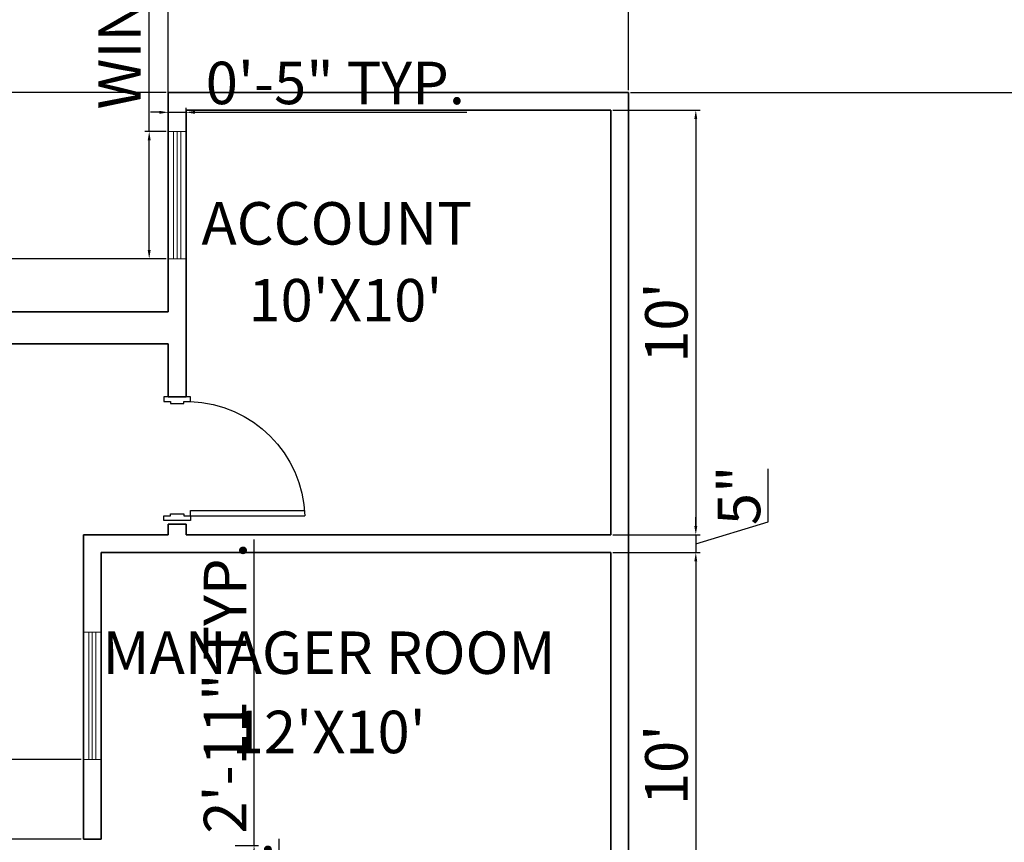
# Model space of a CAD drawing. Units: inches. Extents: x 2319 to 3765, y 2872 to 3950.
# Tile 7 of 9: x 2783 to 3061, y 3357 to 3589. Entities that reach past the tile are written whole.
import ezdxf

# ---------------------------------------------------------------- set-up
doc = ezdxf.new("R2010")
doc.units = ezdxf.units.IN
for name, color, linetype, lineweight in [('A-ANNO-DIMS', 2, 'Continuous', 18), ('A-AREA-IDEN', 7, 'Continuous', 18), ('A-DOOR', 3, 'Continuous', 25), ('A-GLAZ', 4, 'Continuous', 18), ('A-WALL', 7, 'Continuous', 35)]:
    doc.layers.add(name, color=color, linetype=linetype, lineweight=lineweight)
doc.styles.get("Standard").update_dxf_attribs({"font": 'arial.ttf'})
doc.dimstyles.new('ISO-25', dxfattribs={"dimtxt": 12, "dimasz": 2.5, "dimexe": 1.25, "dimexo": 0.625, "dimtad": 1, "dimdec": 0, "dimlunit": 3, "dimtxsty": 'Standard', "dimcen": 2.5, "dimadec": 0, "dimazin": 0, "dimtfac": 1, "dimtdec": 0, "dimtmove": 0, "dimatfit": 3, "dimfxl": 1, "dimarcsym": 0})

# ---------------------------------------------------------------- blocks, each defined once
blk = doc.blocks.new('A$C769D55ED')
for p, q in [((33.6, 192), (33.6, 1024.8)), ((72, 192), (72, 1023.9)), ((0, 192), (0, 0)), ((33.6, 192), (0, 192)), ((33.6, 144), (33.6, 192)), ((48, 144), (33.6, 144)), ((48, 48), (48, 144)), ((33.6, 0), (33.6, 48)), ((33.6, 48), (48, 48)), ((0, 0), (33.6, 0))]:
    blk.add_line(p, q)
blk.add_lwpolyline([(33.6, 192), (72, 192)])
blk.add_lwpolyline([(900, 192), (900, 0), (866.4, 0), (866.4, 48), (852, 48), (852, 144), (866.4, 144), (866.4, 192)], close=True)
blk.add_arc((7.2, 165.6), 859.6, 1.76235, 88.23765)
blk = doc.blocks.new('*D6')
at = {"layer": 'A-ANNO-DIMS', "color": 0, "lineweight": -2, "transparency": 16777216}
for p, q in [((2950.75, 3563.61), (2975.43, 3563.61)), ((2974.18, 3561.11), (2974.18, 3446.11)), ((2950.75, 3443.61), (2975.43, 3443.61))]:
    blk.add_line(p, q, dxfattribs=at)
at = {"layer": 'A-ANNO-DIMS', "color": 0, "transparency": 16777216}
for points in [[(2973.76, 3561.11), (2974.59, 3561.11), (2974.18, 3563.61)], [(2973.76, 3446.11), (2974.59, 3446.11), (2974.18, 3443.61)]]:
    blk.add_solid(points, dxfattribs=at)
at = {"layer": 'Defpoints', "color": 0, "transparency": 16777216}
for p in [(2950.13, 3563.61), (2950.13, 3443.61), (2974.18, 3443.61)]:
    blk.add_point(p, dxfattribs=at)
at = {"layer": 'A-ANNO-DIMS', "color": 0, "transparency": 16777216, "insert": (2967.42, 3503.61), "char_height": 12, "attachment_point": 5, "rotation": 90}
blk.add_mtext("10'", dxfattribs=at)
blk = doc.blocks.new('*D7')
at = {"layer": 'A-ANNO-DIMS', "color": 0, "lineweight": -2, "transparency": 16777216}
for p, q in [((2994.67, 3447.26), (2994.67, 3462.3)), ((2974.18, 3446.11), (2974.18, 3448.61)), ((2974.18, 3441.11), (2994.67, 3447.26)), ((2950.75, 3443.61), (2975.43, 3443.61)), ((2974.18, 3443.61), (2974.18, 3438.61)), ((2974.18, 3443.61), (2974.18, 3438.61)), ((2950.75, 3438.61), (2975.43, 3438.61)), ((2974.18, 3436.11), (2974.18, 3433.61))]:
    blk.add_line(p, q, dxfattribs=at)
at = {"layer": 'A-ANNO-DIMS', "color": 0, "transparency": 16777216}
for points in [[(2973.76, 3446.11), (2974.59, 3446.11), (2974.18, 3443.61)], [(2973.76, 3436.11), (2974.59, 3436.11), (2974.18, 3438.61)]]:
    blk.add_solid(points, dxfattribs=at)
at = {"layer": 'Defpoints', "color": 0, "transparency": 16777216}
for p in [(2950.13, 3443.61), (2950.13, 3438.61), (2974.18, 3438.61)]:
    blk.add_point(p, dxfattribs=at)
at = {"layer": 'A-ANNO-DIMS', "color": 0, "transparency": 16777216, "insert": (2987.94, 3454.78), "char_height": 12, "attachment_point": 5, "rotation": 90}
blk.add_mtext('5"', dxfattribs=at)
blk = doc.blocks.new('*D8')
at = {"layer": 'A-ANNO-DIMS', "color": 0, "lineweight": -2, "transparency": 16777216}
for p, q in [((2950.75, 3438.61), (2975.43, 3438.61)), ((2974.18, 3436.11), (2974.18, 3321.11)), ((2950.75, 3318.61), (2975.43, 3318.61))]:
    blk.add_line(p, q, dxfattribs=at)
at = {"layer": 'A-ANNO-DIMS', "color": 0, "transparency": 16777216}
for points in [[(2973.76, 3436.11), (2974.59, 3436.11), (2974.18, 3438.61)], [(2973.76, 3321.11), (2974.59, 3321.11), (2974.18, 3318.61)]]:
    blk.add_solid(points, dxfattribs=at)
at = {"layer": 'Defpoints', "color": 0, "transparency": 16777216}
for p in [(2950.13, 3438.61), (2950.13, 3318.61), (2974.18, 3318.61)]:
    blk.add_point(p, dxfattribs=at)
at = {"layer": 'A-ANNO-DIMS', "color": 0, "transparency": 16777216, "insert": (2967.42, 3378.61), "char_height": 12, "attachment_point": 5, "rotation": 90}
blk.add_mtext("10'", dxfattribs=at)
blk = doc.blocks.new('WIN-36-PLAN-5IN-WALL')
for p, q in [((0, 36), (5, 36)), ((1.5, 0), (1.5, 36)), ((2.5, 0), (2.5, 36)), ((3.5, 0), (3.5, 36)), ((0, 0), (5, 0))]:
    blk.add_line(p, q)
blk = doc.blocks.new('*D46')
at = {"layer": 'A-ANNO-DIMS', "color": 0, "lineweight": -2, "transparency": 16777216}
for p, q in [((2856.49, 3280.61), (2856.49, 3357.71)), ((2853.02, 3280.61), (2857.74, 3280.61)), ((2856.49, 3259.11), (2856.49, 3278.11)), ((2853.02, 3256.61), (2857.74, 3256.61))]:
    blk.add_line(p, q, dxfattribs=at)
at = {"layer": 'A-ANNO-DIMS', "color": 0, "transparency": 16777216}
for points in [[(2856.07, 3278.11), (2856.91, 3278.11), (2856.49, 3280.61)], [(2856.07, 3259.11), (2856.91, 3259.11), (2856.49, 3256.61)]]:
    blk.add_solid(points, dxfattribs=at)
at = {"layer": 'Defpoints', "color": 0, "transparency": 16777216}
for p in [(2852.39, 3280.61), (2856.49, 3280.61), (2852.39, 3256.61)]:
    blk.add_point(p, dxfattribs=at)
at = {"layer": 'A-ANNO-DIMS', "color": 0, "transparency": 16777216, "insert": (2849.74, 3320.41), "char_height": 12, "attachment_point": 5, "rotation": 90}
blk.add_mtext('2\'-0" TYP.', dxfattribs=at)
blk = doc.blocks.new('*D48')
at = {"layer": 'A-ANNO-DIMS', "color": 0, "lineweight": -2, "transparency": 16777216}
for p, q in [((2849.36, 3355.89), (2849.36, 3442.31)), ((2844.02, 3355.89), (2850.61, 3355.89)), ((2849.36, 3323.46), (2849.36, 3353.39)), ((2844.02, 3320.96), (2850.61, 3320.96))]:
    blk.add_line(p, q, dxfattribs=at)
at = {"layer": 'A-ANNO-DIMS', "color": 0, "transparency": 16777216}
for points in [[(2848.95, 3353.39), (2849.78, 3353.39), (2849.36, 3355.89)], [(2848.95, 3323.46), (2849.78, 3323.46), (2849.36, 3320.96)]]:
    blk.add_solid(points, dxfattribs=at)
at = {"layer": 'Defpoints', "color": 0, "transparency": 16777216}
for p in [(2843.4, 3355.89), (2849.36, 3355.89), (2843.4, 3320.96)]:
    blk.add_point(p, dxfattribs=at)
at = {"layer": 'A-ANNO-DIMS', "color": 0, "transparency": 16777216, "insert": (2842.71, 3400.35), "char_height": 12, "attachment_point": 5, "rotation": 90}
blk.add_mtext('2\'-11" TYP.', dxfattribs=at)
blk = doc.blocks.new('*D61')
at = {"layer": 'A-ANNO-DIMS', "color": 0, "lineweight": -2, "transparency": 16777216}
for p, q in [((2819.73, 3557.62), (2819.73, 3713.22)), ((2824.5, 3557.62), (2818.48, 3557.62)), ((2819.73, 3524.12), (2819.73, 3555.12)), ((2824.5, 3521.62), (2818.48, 3521.62))]:
    blk.add_line(p, q, dxfattribs=at)
at = {"layer": 'A-ANNO-DIMS', "color": 0, "transparency": 16777216}
for points in [[(2819.31, 3555.12), (2820.14, 3555.12), (2819.73, 3557.62)], [(2819.31, 3524.12), (2820.14, 3524.12), (2819.73, 3521.62)]]:
    blk.add_solid(points, dxfattribs=at)
at = {"layer": 'Defpoints', "color": 0, "transparency": 16777216}
for p in [(2819.73, 3557.62), (2825.13, 3557.62), (2825.13, 3521.62)]:
    blk.add_point(p, dxfattribs=at)
at = {"layer": 'A-ANNO-DIMS', "color": 0, "transparency": 16777216, "insert": (2812.89, 3636.67), "char_height": 12, "attachment_point": 5, "rotation": 90}
blk.add_mtext('WINDOW 3\'-0" TYP.', dxfattribs=at)
blk = doc.blocks.new('*D62')
at = {"layer": 'A-ANNO-DIMS', "color": 0, "lineweight": -2, "transparency": 16777216}
for p, q in [((2825.13, 3558.24), (2825.13, 3564.27)), ((2830.13, 3558.24), (2830.13, 3564.27)), ((2822.63, 3563.02), (2820.13, 3563.02)), ((2825.13, 3563.02), (2830.13, 3563.02)), ((2832.63, 3563.02), (2909.52, 3563.02))]:
    blk.add_line(p, q, dxfattribs=at)
at = {"layer": 'A-ANNO-DIMS', "color": 0, "transparency": 16777216}
for points in [[(2822.63, 3563.43), (2822.63, 3562.6), (2825.13, 3563.02)], [(2832.63, 3563.43), (2832.63, 3562.6), (2830.13, 3563.02)]]:
    blk.add_solid(points, dxfattribs=at)
at = {"layer": 'Defpoints', "color": 0, "transparency": 16777216}
for p in [(2830.13, 3563.02), (2825.13, 3557.62), (2830.13, 3557.62)]:
    blk.add_point(p, dxfattribs=at)
at = {"layer": 'A-ANNO-DIMS', "color": 0, "transparency": 16777216, "insert": (2872.32, 3569.77), "char_height": 12, "attachment_point": 5}
blk.add_mtext('0\'-5" TYP.', dxfattribs=at)
blk = doc.blocks.new('*D71')
at = {"layer": 'A-ANNO-DIMS', "color": 0, "lineweight": -2, "transparency": 16777216}
for p, q in [((2474.13, 3507.24), (2474.13, 3605.01)), ((2476.63, 3603.76), (2952.63, 3603.76)), ((2955.13, 3569.24), (2955.13, 3605.01))]:
    blk.add_line(p, q, dxfattribs=at)
at = {"layer": 'A-ANNO-DIMS', "color": 0, "transparency": 16777216}
for points in [[(2476.63, 3604.18), (2476.63, 3603.34), (2474.13, 3603.76)], [(2952.63, 3604.18), (2952.63, 3603.34), (2955.13, 3603.76)]]:
    blk.add_solid(points, dxfattribs=at)
at = {"layer": 'Defpoints', "color": 0, "transparency": 16777216}
for p in [(2955.13, 3603.76), (2955.13, 3568.61), (2474.13, 3506.61)]:
    blk.add_point(p, dxfattribs=at)
at = {"layer": 'A-ANNO-DIMS', "color": 0, "transparency": 16777216, "insert": (2714.63, 3610.51), "char_height": 12, "attachment_point": 5}
blk.add_mtext('40\'-1"', dxfattribs=at)
blk = doc.blocks.new('*D72')
at = {"layer": 'A-ANNO-DIMS', "color": 0, "lineweight": -2, "transparency": 16777216}
for p, q in [((2955.75, 3568.61), (3085.2, 3568.61)), ((3083.95, 2963.11), (3083.95, 3566.11)), ((2955.75, 2960.61), (3085.2, 2960.61))]:
    blk.add_line(p, q, dxfattribs=at)
at = {"layer": 'A-ANNO-DIMS', "color": 0, "transparency": 16777216}
for points in [[(3083.53, 3566.11), (3084.36, 3566.11), (3083.95, 3568.61)], [(3083.53, 2963.11), (3084.36, 2963.11), (3083.95, 2960.61)]]:
    blk.add_solid(points, dxfattribs=at)
at = {"layer": 'Defpoints', "color": 0, "transparency": 16777216}
for p in [(2955.13, 3568.61), (3083.95, 3568.61), (2955.13, 2960.61)]:
    blk.add_point(p, dxfattribs=at)
at = {"layer": 'A-ANNO-DIMS', "color": 0, "transparency": 16777216, "insert": (3077.2, 3264.61), "char_height": 12, "attachment_point": 5, "rotation": 90}
blk.add_mtext('50\'-8"', dxfattribs=at)
blk = doc.blocks.new('*D73')
at = {"layer": 'A-ANNO-DIMS', "color": 0, "lineweight": -2, "transparency": 16777216}
for p, q in [((2474.13, 3507.24), (2474.13, 3605.01)), ((2476.63, 3603.76), (2822.63, 3603.76)), ((2825.13, 3507.24), (2825.13, 3605.01))]:
    blk.add_line(p, q, dxfattribs=at)
at = {"layer": 'A-ANNO-DIMS', "color": 0, "transparency": 16777216}
for points in [[(2476.63, 3604.18), (2476.63, 3603.34), (2474.13, 3603.76)], [(2822.63, 3604.18), (2822.63, 3603.34), (2825.13, 3603.76)]]:
    blk.add_solid(points, dxfattribs=at)
at = {"layer": 'Defpoints', "color": 0, "transparency": 16777216}
for p in [(2825.13, 3603.76), (2474.13, 3506.61), (2825.13, 3506.61)]:
    blk.add_point(p, dxfattribs=at)
at = {"layer": 'A-ANNO-DIMS', "color": 0, "transparency": 16777216, "insert": (2649.63, 3610.52), "char_height": 12, "attachment_point": 5}
blk.add_mtext('29\'-3"', dxfattribs=at)
blk = doc.blocks.new('*D74')
at = {"layer": 'A-ANNO-DIMS', "color": 0, "lineweight": -2, "transparency": 16777216}
for p, q in [((2824.5, 3568.61), (2341.89, 3568.61)), ((2343.14, 3509.11), (2343.14, 3566.11)), ((2824.5, 3506.61), (2341.89, 3506.61))]:
    blk.add_line(p, q, dxfattribs=at)
at = {"layer": 'A-ANNO-DIMS', "color": 0, "transparency": 16777216}
for points in [[(2342.72, 3566.11), (2343.56, 3566.11), (2343.14, 3568.61)], [(2342.72, 3509.11), (2343.56, 3509.11), (2343.14, 3506.61)]]:
    blk.add_solid(points, dxfattribs=at)
at = {"layer": 'Defpoints', "color": 0, "transparency": 16777216}
for p in [(2343.14, 3568.61), (2825.13, 3568.61), (2825.13, 3506.61)]:
    blk.add_point(p, dxfattribs=at)
at = {"layer": 'A-ANNO-DIMS', "color": 0, "transparency": 16777216, "insert": (2336.39, 3537.61), "char_height": 12, "attachment_point": 5, "rotation": 90}
blk.add_mtext('5\'-2"', dxfattribs=at)
blk = doc.blocks.new('*D76')
at = {"layer": 'A-ANNO-DIMS', "color": 0, "lineweight": -2, "transparency": 16777216}
for p, q in [((2757.13, 2970.24), (2757.13, 3605.01)), ((2759.63, 3603.76), (2773.17, 3603.76)), ((2775.67, 2970.24), (2775.67, 3605.01)), ((2775.67, 3603.76), (2838.15, 3603.76))]:
    blk.add_line(p, q, dxfattribs=at)
at = {"layer": 'A-ANNO-DIMS', "color": 0, "transparency": 16777216}
for points in [[(2759.63, 3604.18), (2759.63, 3603.34), (2757.13, 3603.76)], [(2773.17, 3604.18), (2773.17, 3603.34), (2775.67, 3603.76)]]:
    blk.add_solid(points, dxfattribs=at)
at = {"layer": 'Defpoints', "color": 0, "transparency": 16777216}
for p in [(2775.67, 3603.76), (2757.13, 2969.61), (2775.67, 2969.61)]:
    blk.add_point(p, dxfattribs=at)
at = {"layer": 'A-ANNO-DIMS', "color": 0, "transparency": 16777216, "insert": (2808.16, 3610.59), "char_height": 12, "attachment_point": 5}
blk.add_mtext('1\'-6 1/2"', dxfattribs=at)
blk = doc.blocks.new('*D86')
at = {"layer": 'A-ANNO-DIMS', "color": 0, "lineweight": -2, "transparency": 16777216}
for p, q in [((2343.14, 3521.62), (2343.14, 3556.13)), ((2824.5, 3521.62), (2341.89, 3521.62)), ((2343.14, 3509.11), (2343.14, 3519.12)), ((2824.5, 3506.61), (2341.89, 3506.61))]:
    blk.add_line(p, q, dxfattribs=at)
at = {"layer": 'A-ANNO-DIMS', "color": 0, "transparency": 16777216}
for points in [[(2342.72, 3519.12), (2343.56, 3519.12), (2343.14, 3521.62)], [(2342.72, 3509.11), (2343.56, 3509.11), (2343.14, 3506.61)]]:
    blk.add_solid(points, dxfattribs=at)
at = {"layer": 'Defpoints', "color": 0, "transparency": 16777216}
for p in [(2343.14, 3521.62), (2825.13, 3521.62), (2825.13, 3506.61)]:
    blk.add_point(p, dxfattribs=at)
at = {"layer": 'A-ANNO-DIMS', "color": 0, "transparency": 16777216, "insert": (2336.38, 3540.13), "char_height": 12, "attachment_point": 5, "rotation": 90}
blk.add_mtext('1\'-3"', dxfattribs=at)
blk = doc.blocks.new('*D87')
at = {"layer": 'A-ANNO-DIMS', "color": 0, "lineweight": -2, "transparency": 16777216}
for p, q in [((2800.5, 3380.11), (2341.89, 3380.11)), ((2343.14, 3377.61), (2343.14, 3360.11)), ((2800.5, 3357.61), (2341.89, 3357.61)), ((2343.14, 3357.61), (2343.14, 3285.81))]:
    blk.add_line(p, q, dxfattribs=at)
at = {"layer": 'A-ANNO-DIMS', "color": 0, "transparency": 16777216}
for points in [[(2342.72, 3377.61), (2343.56, 3377.61), (2343.14, 3380.11)], [(2342.72, 3360.11), (2343.56, 3360.11), (2343.14, 3357.61)]]:
    blk.add_solid(points, dxfattribs=at)
at = {"layer": 'Defpoints', "color": 0, "transparency": 16777216}
for p in [(2801.13, 3380.11), (2343.14, 3357.61), (2801.13, 3357.61)]:
    blk.add_point(p, dxfattribs=at)
at = {"layer": 'A-ANNO-DIMS', "color": 0, "transparency": 16777216, "insert": (2336.31, 3320.46), "char_height": 12, "attachment_point": 5, "rotation": 90}
blk.add_mtext('1\'-10 1/2"', dxfattribs=at)

msp = doc.modelspace()

# ---------------------------------------------------------------- linework, layer by layer
at = {"layer": 'A-WALL'}
for p, q in [((2955.13, 3568.61), (2825.13, 3568.61)), ((2825.13, 3506.61), (2825.13, 3568.61)), ((2955.13, 3443.61), (2955.13, 3568.61)), ((2950.13, 3563.61), (2830.13, 3563.61)), ((2830.13, 3482.61), (2830.13, 3563.61)), ((2950.13, 3443.61), (2950.13, 3563.61)), ((2474.13, 3506.61), (2825.13, 3506.61)), ((2608.13, 3497.61), (2825.13, 3497.61)), ((2825.13, 3482.61), (2825.13, 3497.61)), ((2830.13, 3482.61), (2825.13, 3482.61)), ((2825.13, 3443.61), (2825.13, 3446.61)), ((2830.13, 3446.61), (2825.13, 3446.61)), ((2830.13, 3443.61), (2830.13, 3446.61)), ((2801.13, 3443.61), (2801.13, 3357.61)), ((2825.13, 3443.61), (2801.13, 3443.61)), ((2950.13, 3443.61), (2830.13, 3443.61)), ((2955.13, 3248.61), (2955.13, 3443.61)), ((2950.13, 3438.61), (2806.13, 3438.61)), ((2806.13, 3438.61), (2806.13, 3357.61)), ((2950.13, 3318.61), (2950.13, 3438.61)), ((2806.13, 3357.61), (2801.13, 3357.61))]:
    msp.add_line(p, q, dxfattribs=at)

# ---------------------------------------------------------------- block references
at = {"layer": 'A-DOOR', "xscale": -0.0388089662083284, "yscale": 0.0388089662083284, "zscale": 0.0388089662083284, "rotation": 270}
msp.add_blockref('A$C769D55ED', (2823.9, 3447.68), dxfattribs=at)
at = {"layer": 'A-GLAZ'}
for p in [(2825.13, 3521.62), (2801.13, 3380.11)]:
    msp.add_blockref('WIN-36-PLAN-5IN-WALL', p, dxfattribs=at)

# ---------------------------------------------------------------- texts
at = {"layer": 'A-AREA-IDEN'}
for s, p in [('ACCOUNT ', (2834.5, 3525.64)), ("10'X10'", (2847.76, 3503.93)), ('MANAGER ROOM', (2806.54, 3404.32)), ("12'X10'", (2843.06, 3381.93))]:
    msp.add_text(s, height=12, dxfattribs=at).set_placement(p)

# ---------------------------------------------------------------- dimensions: what is measured, and where the dimension line sits
at = {"layer": 'A-ANNO-DIMS'}
for base, p1, p2, text, picture, middle in [((2819.73, 3557.62), (2825.13, 3521.62), (2825.13, 3557.62), 'WINDOW <> TYP.', '*D61', (2812.89, 3636.67)), ((2849.36, 3355.89), (2843.4, 3320.96), (2843.4, 3355.89), '<> TYP.', '*D48', (2842.71, 3400.35)), ((2856.49, 3280.61), (2852.39, 3256.61), (2852.39, 3280.61), '<> TYP.', '*D46', (2849.74, 3320.41))]:
    dim = msp.add_linear_dim(base=base, p1=p1, p2=p2, angle=90, text=text, dimstyle='ISO-25', override={"dimdec": 1, "dimlfac": 1, "dimrnd": 0, "dimzin": 1, "dimdsep": 46, "dimlunit": 4, "dimfrac": 2}, dxfattribs=at)
    dim.commit()
    dim.dimension.update_dxf_attribs({"geometry": picture, "text_midpoint": middle})
for base, p1, p2, picture, middle in [((2775.67, 3603.76), (2757.13, 2969.61), (2775.67, 2969.61), '*D76', (2808.16, 3610.59)), ((2955.13, 3603.76), (2474.13, 3506.61), (2955.13, 3568.61), '*D71', (2714.63, 3610.51)), ((2825.13, 3603.76), (2474.13, 3506.61), (2825.13, 3506.61), '*D73', (2649.63, 3610.52))]:
    dim = msp.add_linear_dim(base=base, p1=p1, p2=p2, dimstyle='ISO-25', override={"dimdec": 1, "dimlfac": 1, "dimrnd": 0, "dimzin": 1, "dimdsep": 46, "dimlunit": 4, "dimfrac": 2}, dxfattribs=at)
    dim.commit()
    dim.dimension.update_dxf_attribs({"geometry": picture, "text_midpoint": middle})
dim = msp.add_linear_dim(base=(2830.13, 3563.02), p1=(2825.13, 3557.62), p2=(2830.13, 3557.62), text='<> TYP.', dimstyle='ISO-25', override={"dimdec": 1, "dimlfac": 1, "dimrnd": 0, "dimzin": 1, "dimdsep": 46, "dimlunit": 4, "dimfrac": 2}, dxfattribs=at)
dim.commit()
dim.dimension.update_dxf_attribs({"geometry": '*D62', "text_midpoint": (2872.32, 3569.77)})
for base, p1, p2, override, picture, middle in [((2343.14, 3568.61), (2825.13, 3506.61), (2825.13, 3568.61), {"dimdec": 1, "dimlfac": 1, "dimrnd": 0, "dimzin": 1, "dimdsep": 46, "dimlunit": 4, "dimfrac": 2}, '*D74', (2336.39, 3537.61)), ((3083.95, 3568.61), (2955.13, 2960.61), (2955.13, 3568.61), {"dimdec": 1, "dimlfac": 1, "dimrnd": 0, "dimzin": 1, "dimdsep": 46, "dimlunit": 4, "dimfrac": 2}, '*D72', (3077.2, 3264.61)), ((2974.18, 3443.61), (2950.13, 3563.61), (2950.13, 3443.61), {"dimclrd": 0, "dimclre": 0, "dimclrt": 0}, '*D6', (2967.42, 3503.61)), ((2343.14, 3521.62), (2825.13, 3506.61), (2825.13, 3521.62), {"dimdec": 1, "dimlfac": 1, "dimrnd": 0, "dimzin": 1, "dimdsep": 46, "dimlunit": 4, "dimfrac": 2}, '*D86', (2336.38, 3540.13)), ((2974.18, 3438.61), (2950.13, 3443.61), (2950.13, 3438.61), {"dimclrd": 0, "dimclre": 0, "dimclrt": 0, "dimtmove": 1}, '*D7', (2987.94, 3447.88)), ((2974.18, 3318.61), (2950.13, 3438.61), (2950.13, 3318.61), {"dimclrd": 0, "dimclre": 0, "dimclrt": 0, "dimtmove": 1}, '*D8', (2967.42, 3378.61)), ((2343.14, 3357.61), (2801.13, 3380.11), (2801.13, 3357.61), {"dimdec": 1, "dimlfac": 1, "dimrnd": 0, "dimzin": 1, "dimdsep": 46, "dimlunit": 4, "dimfrac": 2}, '*D87', (2336.31, 3320.46))]:
    dim = msp.add_linear_dim(base=base, p1=p1, p2=p2, angle=90, dimstyle='ISO-25', override=override, dxfattribs=at)
    dim.commit()
    dim.dimension.update_dxf_attribs({"geometry": picture, "text_midpoint": middle})

doc.saveas('drawing.dxf')
